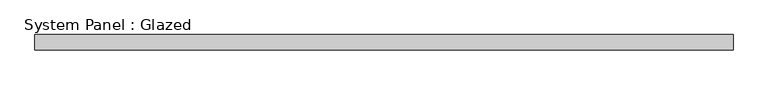
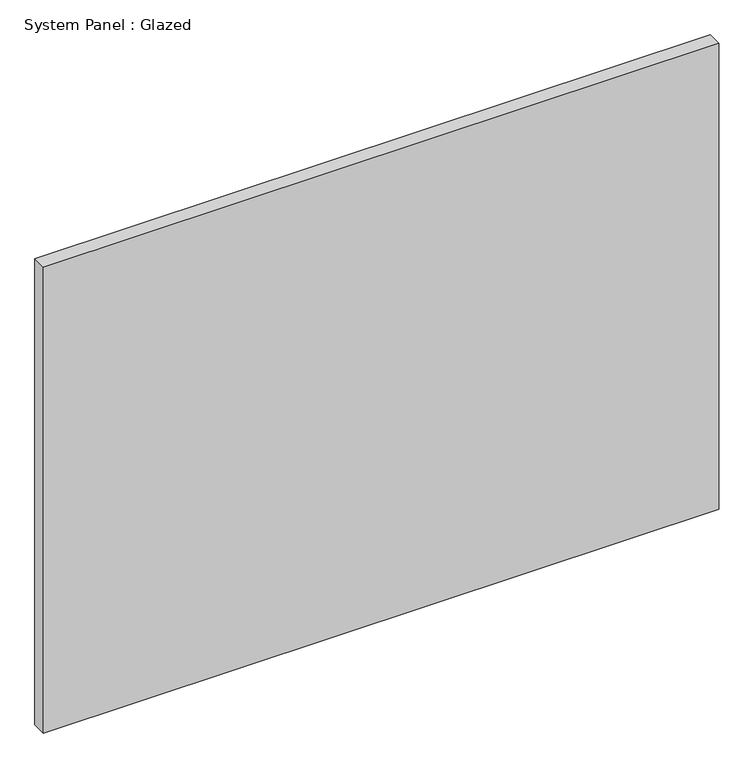
"""IFC4 building model written with IfcOpenShell, lengths in millimetres: plate geometry, System Panel : Glazed."""

from ifc_helpers import new_model, si_unit, origin, origin_with_axes, place, context, project, spatial, polyline, outline, extrude, source, transform, mapped, element, save


def system_panel_glazed_3e9834e9(model_context):
    return source(origin(), model_context, "Body", "SweptSolid", [
        extrude(outline(polyline([(581.0249999, 19.05), (-581.0249999, 19.05), (-581.0249999, 44.45), (581.0249999, 44.45), (581.0249999, 19.05)])), origin_with_axes(), (0.0, 0.0, 1.0), 847.5210507),
    ])


if __name__ == "__main__":
    model = new_model("IFC4")
    model_context = context("Model", 3, world=origin())
    ifc_project = project(units=[si_unit("LENGTHUNIT", "METRE", prefix="MILLI")], contexts=[model_context])
    site = spatial("IfcSite", under=ifc_project)
    building = spatial("IfcBuilding", under=site)
    placement = place(None, origin())
    system_panel_glazed_shape = system_panel_glazed_3e9834e9(model_context)
    element("IfcPlate", 1, ObjectType="System Panel : Glazed", at=placement, inside=building, context=model_context, shape_type="MappedRepresentation", body=[
        mapped(system_panel_glazed_shape, transform((0.0, 0.0, 0.0), x_axis=(1.0, 0.0, 0.0), y_axis=(0.0, 1.0, 0.0), z_axis=(0.0, 0.0, 1.0))),
    ])
    save(model, "model.ifc")

# Revit data of these elements
# Type "System Panel : Glazed"
#   Construction Type Id = "GSP4R"
#   Analytic Construction = "1/8 in Pilkington single glazing"
#   Visual Light Transmittance = 0.9
#   Solar Heat Gain Coefficient = 0.86
#   Heat Transfer Coefficient (U) = 1.18115 BTU/(h·ft²·°F)
#   Define Thermal Properties by = 1
# Element 1 (IfcPlate, "System Panel : Glazed")
#   Materials on its faces: "Glass"
# Materials
#   "Glass": class "Glass", colour RGB 0 128 192, transparency 0.75, Description = "Soda Lime Glass", Cost = 0
